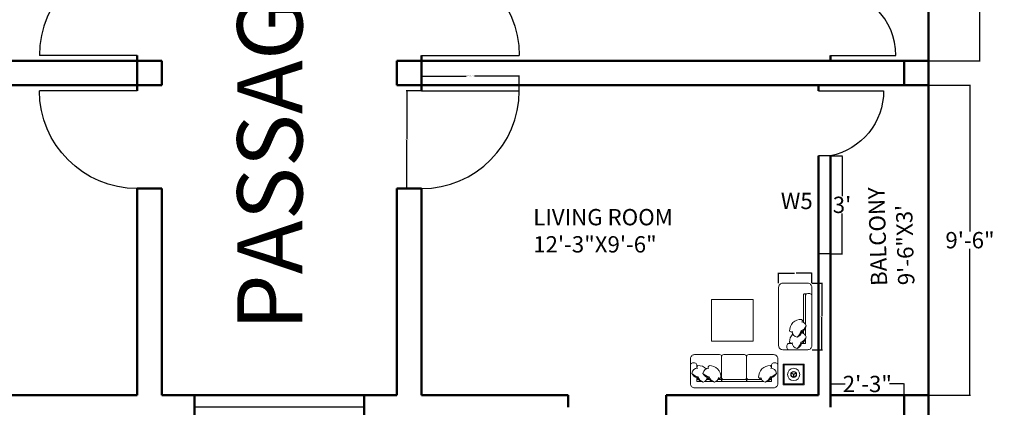
# Model space of a CAD drawing. Units: inches. Extents: x -173 to 545, y -746 to 104.
# Tile 20 of 32: x 168 to 530, y -463 to -321. Entities that reach past the tile are written whole.
import ezdxf

# ---------------------------------------------------------------- set-up
doc = ezdxf.new("R2010")
doc.units = ezdxf.units.IN
doc.header["$MEASUREMENT"] = 0
for name, color, linetype, lineweight in [('A-ANNO-DIMS', 2, 'Continuous', 18), ('A-ANNO-TEXT', 7, 'Continuous', 18), ('A-AREA-IDEN', 7, 'Continuous', 18), ('A-DOOR', 4, 'Continuous', 25), ('A-FURN', 8, 'Continuous', 18), ('A-GLAZ', 3, 'Continuous', 25), ('A-WALL', 7, 'Continuous', 50)]:
    doc.layers.add(name, color=color, linetype=linetype, lineweight=lineweight)
doc.styles.get("Standard").update_dxf_attribs({"font": 'arial.ttf'})
doc.dimstyles.get("Standard").update_dxf_attribs({"dimtxt": 0.18, "dimasz": 0.18, "dimexe": 0.18, "dimexo": 0.0625, "dimgap": 0.09, "dimtad": 0, "dimtih": 1, "dimtoh": 1, "dimdec": 0, "dimzin": 0, "dimdsep": 46, "dimlunit": 3, "dimtxsty": 'Standard', "dimcen": 0.09, "dimadec": 0, "dimazin": 0, "dimtfac": 1, "dimtdec": 0, "dimtofl": 0, "dimtmove": 0, "dimatfit": 3, "dimfxl": 1, "dimtolj": 1, "dimtzin": 0, "dimarcsym": 0})

# ---------------------------------------------------------------- blocks, each defined once
blk = doc.blocks.new('*D8')
at = {"layer": 'A-ANNO-DIMS', "color": 0, "lineweight": -2, "transparency": 16777216}
for p, q in [((501.86, -221.86), (520.82, -221.86)), ((520.64, -222.04), (520.64, -275.71)), ((520.64, -335.68), (520.64, -282.02)), ((501.86, -335.86), (520.82, -335.86))]:
    blk.add_line(p, q, dxfattribs=at)
at = {"layer": 'A-ANNO-DIMS', "color": 0, "transparency": 16777216}
for points in [[(520.61, -222.04), (520.67, -222.04), (520.64, -221.86)], [(520.61, -335.68), (520.67, -335.68), (520.64, -335.86)]]:
    blk.add_solid(points, dxfattribs=at)
at = {"layer": 'Defpoints', "color": 0, "transparency": 16777216}
for p in [(501.8, -221.86), (501.8, -335.86), (520.64, -335.86)]:
    blk.add_point(p, dxfattribs=at)
at = {"layer": 'A-ANNO-DIMS', "color": 0, "transparency": 16777216, "insert": (520.64, -278.86), "char_height": 6, "attachment_point": 5}
blk.add_mtext('\\A1;9\'-6"', dxfattribs=at)
blk = doc.blocks.new('*D13')
at = {"layer": 'A-ANNO-DIMS', "color": 0, "lineweight": -2, "transparency": 16777216}
for p, q in [((465.86, -370.86), (470.17, -370.86)), ((469.99, -371.04), (469.99, -385.71)), ((469.99, -406.68), (469.99, -392.02)), ((465.86, -406.86), (470.17, -406.86))]:
    blk.add_line(p, q, dxfattribs=at)
at = {"layer": 'A-ANNO-DIMS', "color": 0, "transparency": 16777216}
for points in [[(469.96, -371.04), (470.02, -371.04), (469.99, -370.86)], [(469.96, -406.68), (470.02, -406.68), (469.99, -406.86)]]:
    blk.add_solid(points, dxfattribs=at)
at = {"layer": 'Defpoints', "color": 0, "transparency": 16777216}
for p in [(465.8, -370.86), (465.8, -406.86), (469.99, -406.86)]:
    blk.add_point(p, dxfattribs=at)
at = {"layer": 'A-ANNO-DIMS', "color": 0, "transparency": 16777216, "insert": (469.99, -388.86), "char_height": 6, "attachment_point": 5}
blk.add_mtext("\\A1;3'", dxfattribs=at)
blk = doc.blocks.new('*D17')
at = {"layer": 'A-ANNO-DIMS', "color": 0, "lineweight": -2, "transparency": 16777216}
for p, q in [((465.8, -458.8), (465.8, -454.59)), ((465.98, -454.77), (471.19, -454.77)), ((492.62, -454.77), (487.42, -454.77)), ((492.8, -458.8), (492.8, -454.59))]:
    blk.add_line(p, q, dxfattribs=at)
at = {"layer": 'A-ANNO-DIMS', "color": 0, "transparency": 16777216}
for points in [[(465.98, -454.74), (465.98, -454.8), (465.8, -454.77)], [(492.62, -454.74), (492.62, -454.8), (492.8, -454.77)]]:
    blk.add_solid(points, dxfattribs=at)
at = {"layer": 'Defpoints', "color": 0, "transparency": 16777216}
for p in [(492.8, -454.77), (465.8, -458.86), (492.8, -458.86)]:
    blk.add_point(p, dxfattribs=at)
at = {"layer": 'A-ANNO-DIMS', "color": 0, "transparency": 16777216, "insert": (479.3, -454.77), "char_height": 6, "attachment_point": 5}
blk.add_mtext('\\A1;2\'-3"', dxfattribs=at)
blk = doc.blocks.new('*D18')
at = {"layer": 'A-ANNO-DIMS', "color": 0, "lineweight": -2, "transparency": 16777216}
for p, q in [((501.86, -344.86), (517.24, -344.86)), ((517.06, -345.04), (517.06, -398.71)), ((517.06, -458.68), (517.06, -405.02)), ((501.86, -458.86), (517.24, -458.86))]:
    blk.add_line(p, q, dxfattribs=at)
at = {"layer": 'A-ANNO-DIMS', "color": 0, "transparency": 16777216}
for points in [[(517.03, -345.04), (517.09, -345.04), (517.06, -344.86)], [(517.03, -458.68), (517.09, -458.68), (517.06, -458.86)]]:
    blk.add_solid(points, dxfattribs=at)
at = {"layer": 'Defpoints', "color": 0, "transparency": 16777216}
for p in [(501.8, -344.86), (501.8, -458.86), (517.06, -458.86)]:
    blk.add_point(p, dxfattribs=at)
at = {"layer": 'A-ANNO-DIMS', "color": 0, "transparency": 16777216, "insert": (517.06, -401.86), "char_height": 6, "attachment_point": 5}
blk.add_mtext('\\A1;9\'-6"', dxfattribs=at)
blk = doc.blocks.new('DAY BED1')
at = {"color": 0}
blk.add_line((0.3, 0.25), (0.225, 0.255), dxfattribs=at)
blk.add_lwpolyline([(-0.3, 0, -0.414214), (-0.4, 0.1), (-0.4, 0.1, 0.317837), (-0.4, 0.1, -0.414214), (-0.4, 0.1), (-0.4, 0.1, 1.186185), (-0.4, 0.1, -0.414214), (-0.4, 0.1), (-0.4, 1.5, -0.414214), (-0.3, 1.6), (0.3, 1.6, -0.414214), (0.4, 1.5), (0.4, 0.1, -0.414214), (0.3, 0)], format="xyb", close=True, dxfattribs=at)
for points in [[(-0.073, 1.45), (-0.15, 1.45, -0.414214), (-0.2, 1.5), (-0.2, 1.55, -0.414214), (-0.15, 1.6)], [(-0.073, 1.45, 0.165541), (-0.139, 1.419, 0.200231), (-0.058, 1.221, 0.121523)], [(-0.076, 1.425, -0.356772), (0.05, 1.568, -0.249542), (0.154, 1.438, 9.61688)], [(0.05, 1.568, -0.14773), (0.136, 1.422, -0.213343), (0.262, 1.293, -0.178662)], [(0.143, 1.442, -0.306663), (0.262, 1.293, -0.30633), (0.154, 1.196, 0.872847)], [(0.25, 1.345), (0.25, 1.45), (0.152, 1.45, -0.414214)], [(0.2, 1.412), (0.2, 1.43, -0.414214), (0.22, 1.45), (0.23, 1.45, -0.414214), (0.25, 1.43)], [(0.25, 1.43), (0.25, 1.345, -0.414214)], [(-0.076, 1.156, -0.356772), (0.05, 1.299, -0.249542), (0.154, 1.169, 9.61688)], [(0.05, 1.299, -0.14773), (0.136, 1.153, -0.213343), (0.262, 1.024, -0.178662)], [(0.168, 1.163, 0.071865), (0.187, 1.205, -7.115464)], [(0.2, 1.142), (0.2, 1.211, -0.414214)], [(0.25, 1.262), (0.25, 1.075, -0.414214)], [(-0.073, 1.181, 0.165541), (-0.139, 1.15, 0.425989), (0.148, 0.869, 0.121523), (0.187, 0.936, -7.115464)], [(0.143, 1.173, -0.306663), (0.262, 1.024, -0.30633), (0.154, 0.926, 0.872847)], [(0.25, 0.992), (0.25, 0.275, -0.414214), (0.23, 0.255), (0.22, 0.255, -0.414214), (0.2, 0.275), (0.2, 0.942, -0.414214)], [(0.25, 0.377), (0.25, 0.3, 0.414214), (0.3, 0.25), (0.35, 0.25, 0.414214), (0.4, 0.3)]]:
    blk.add_lwpolyline(points, format="xyb", dxfattribs=at)
for points in [[(0.25, 1.075), (0.25, 1.262)], [(0.25, 0.377), (0.25, 0.992)]]:
    blk.add_lwpolyline(points, dxfattribs=at)
blk = doc.blocks.new('DOOR-24')
blk.add_line((24, 0), (24, 24))
blk.add_arc((24, 0), 24, 90, 180)
blk = doc.blocks.new('DOOR-36')
blk.add_line((36, 0), (0, 0))
blk.add_arc((36, 0), 36, 90, 180)
blk = doc.blocks.new('DOOR-24-OFFSET')
blk.add_line((24, 24), (0, 24))
blk.add_arc((24.52, 24), 24.52, 180, 258.1877)
blk = doc.blocks.new('*D50')
at = {"layer": 'A-ANNO-DIMS', "color": 0, "lineweight": -2, "transparency": 16777216}
for p, q in [((458.97, -417.69), (462.76, -417.69)), ((462.58, -417.87), (462.58, -429.75)), ((462.58, -442), (462.58, -430.12)), ((458.97, -442.18), (462.76, -442.18))]:
    blk.add_line(p, q, dxfattribs=at)
at = {"layer": 'A-ANNO-DIMS', "color": 0, "transparency": 16777216}
for points in [[(462.55, -417.87), (462.61, -417.87), (462.58, -417.69)], [(462.55, -442), (462.61, -442), (462.58, -442.18)]]:
    blk.add_solid(points, dxfattribs=at)
at = {"layer": 'Defpoints', "color": 0, "transparency": 16777216}
for p in [(458.91, -417.69), (458.91, -442.18), (462.58, -442.18)]:
    blk.add_point(p, dxfattribs=at)
at = {"layer": 'A-ANNO-DIMS', "color": 0, "transparency": 16777216, "insert": (462.58, -429.94), "char_height": 0.18, "attachment_point": 5}
blk.add_mtext('\\A1;DAY BED 2\'-0 1/2"', dxfattribs=at)
blk = doc.blocks.new('*D51')
at = {"layer": 'A-ANNO-DIMS', "color": 0, "lineweight": -2, "transparency": 16777216}
for p, q in [((446.67, -417.63), (446.67, -413.84)), ((446.85, -414.02), (452.47, -414.02)), ((458.73, -414.02), (453.11, -414.02)), ((458.91, -417.63), (458.91, -413.84))]:
    blk.add_line(p, q, dxfattribs=at)
at = {"layer": 'A-ANNO-DIMS', "color": 0, "transparency": 16777216}
for points in [[(446.85, -413.99), (446.85, -414.05), (446.67, -414.02)], [(458.73, -413.99), (458.73, -414.05), (458.91, -414.02)]]:
    blk.add_solid(points, dxfattribs=at)
at = {"layer": 'Defpoints', "color": 0, "transparency": 16777216}
for p in [(458.91, -414.02), (446.67, -417.69), (458.91, -417.69)]:
    blk.add_point(p, dxfattribs=at)
at = {"layer": 'A-ANNO-DIMS', "color": 0, "transparency": 16777216, "insert": (452.79, -414.02), "char_height": 0.18, "attachment_point": 5}
blk.add_mtext('\\A1;1\'-0"', dxfattribs=at)
blk = doc.blocks.new('*D54')
at = {"layer": 'A-ANNO-DIMS', "color": 0, "lineweight": -2, "transparency": 16777216}
for p, q in [((315.3, -346.8), (315.3, -341.28)), ((315.48, -341.46), (331.79, -341.46)), ((351.12, -341.46), (334.81, -341.46)), ((351.3, -346.8), (351.3, -341.28))]:
    blk.add_line(p, q, dxfattribs=at)
at = {"layer": 'A-ANNO-DIMS', "color": 0, "transparency": 16777216}
for points in [[(315.48, -341.43), (315.48, -341.49), (315.3, -341.46)], [(351.12, -341.43), (351.12, -341.49), (351.3, -341.46)]]:
    blk.add_solid(points, dxfattribs=at)
at = {"layer": 'Defpoints', "color": 0, "transparency": 16777216}
for p in [(315.3, -341.46), (315.3, -346.86), (351.3, -346.86)]:
    blk.add_point(p, dxfattribs=at)
at = {"layer": 'A-ANNO-DIMS', "color": 0, "transparency": 16777216, "insert": (333.3, -341.46), "char_height": 0.18, "attachment_point": 5}
blk.add_mtext('\\A1;ENTRY DOOR 3\'-0" TYP.', dxfattribs=at)
blk = doc.blocks.new('*D55')
at = {"layer": 'A-ANNO-DIMS', "color": 0, "lineweight": -2, "transparency": 16777216}
for p, q in [((315.24, -346.86), (309.72, -346.86)), ((309.9, -347.04), (309.9, -364.68)), ((309.9, -382.68), (309.9, -365.04)), ((315.24, -382.86), (309.72, -382.86))]:
    blk.add_line(p, q, dxfattribs=at)
at = {"layer": 'A-ANNO-DIMS', "color": 0, "transparency": 16777216}
for points in [[(309.87, -347.04), (309.93, -347.04), (309.9, -346.86)], [(309.87, -382.68), (309.93, -382.68), (309.9, -382.86)]]:
    blk.add_solid(points, dxfattribs=at)
at = {"layer": 'Defpoints', "color": 0, "transparency": 16777216}
for p in [(315.3, -346.86), (309.9, -382.86), (315.3, -382.86)]:
    blk.add_point(p, dxfattribs=at)
at = {"layer": 'A-ANNO-DIMS', "color": 0, "transparency": 16777216, "insert": (309.9, -364.86), "char_height": 0.18, "attachment_point": 5}
blk.add_mtext('\\A1;3\'-0" TYP.', dxfattribs=at)

msp = doc.modelspace()

# ---------------------------------------------------------------- linework, layer by layer
at = {"layer": 'A-DOOR'}
msp.add_line((294.3, -463.36), (231.8, -463.36), dxfattribs=at)
at = {"layer": 'A-FURN'}
for p, q in [((452.19, -451.3), (451.26, -450.76)), ((452.24, -451.21), (451.3, -450.67)), ((452.17, -451.26), (452.17, -452.33)), ((452.19, -451.21), (453.12, -450.67)), ((452.24, -451.3), (453.17, -450.76)), ((452.26, -451.26), (452.26, -452.33))]:
    msp.add_line(p, q, dxfattribs=at)
at = {"layer": 'A-FURN', "ltscale": 0.03}
for points in [[(421.99, -423.71), (437.3, -423.71), (437.3, -439.01), (421.99, -439.01)], [(456.04, -447.43), (448.39, -447.43), (448.39, -455.08), (456.04, -455.08)]]:
    msp.add_lwpolyline(points, close=True, dxfattribs=at)
msp.add_lwpolyline([(446.38, -445.5, 0.414214), (444.85, -443.97), (435.67, -443.97, 0.414214), (434.9, -444.73, 0.414214), (434.14, -443.97), (426.49, -443.97, 0.414214), (425.72, -444.73, 0.414214), (424.96, -443.97), (415.78, -443.97, 0.414214), (414.25, -445.5), (414.25, -454.68, 0.414214), (415.78, -456.21), (444.85, -456.21, 0.414214), (446.38, -454.68)], format="xyb", close=True, dxfattribs=at)
at = {"layer": 'A-FURN'}
for points in [[(424.96, -453.15, 0.414214), (425.72, -452.38), (425.72, -444.73, 0.414214)], [(435.67, -453.15, -0.414214), (434.9, -452.38), (434.9, -444.73, -0.414214)], [(416.54, -448.98), (416.54, -447.79, 0.414214), (415.78, -447.03), (415.01, -447.03, 0.414214), (414.25, -447.79)], [(416.92, -448.93, 0.356772), (414.73, -450.86, 0.249542), (416.72, -452.45, -9.61688)], [(416.54, -448.98, -0.165541), (417.01, -447.97, -0.200231), (420.05, -449.2, -0.121523)], [(421.05, -448.93, 0.356772), (418.85, -450.86, 0.249542), (420.84, -452.45, -9.61688)], [(420.66, -448.98, -0.165541), (421.13, -447.97, -0.425989), (425.43, -452.35, -0.121523), (424.41, -452.95, 7.115464)], [(444.09, -448.98, 0.165541), (443.61, -447.97, 0.425989), (439.32, -452.35, 0.121523), (440.34, -452.95, -7.115464)], [(443.7, -448.93, -0.356772), (445.89, -450.86, -0.249542), (443.91, -452.45, 9.61688)], [(446.38, -447.79, 0.414214), (445.61, -447.03), (444.85, -447.03, 0.414214), (444.08, -447.79), (444.08, -448.98)], [(414.73, -450.86, 0.14773), (416.97, -452.17, 0.213343), (418.94, -454.1, 0.178662)], [(418.15, -453.91), (416.54, -453.91), (416.54, -452.41, 0.414214)], [(416.66, -452.28, 0.306663), (418.94, -454.1, 0.30633), (420.43, -452.44, -0.872847)], [(418.85, -450.86, 0.14773), (421.09, -452.17, 0.213343), (423.06, -454.1, 0.178662)], [(420.93, -452.65, -0.071865), (420.29, -452.95, 7.115464)], [(420.78, -452.28, 0.306663), (423.06, -454.1, 0.30633), (424.55, -452.44, -0.872847)], [(426.49, -453.15, -0.414214), (425.72, -452.38)], [(434.14, -453.15, 0.414214), (434.9, -452.38)], [(443.96, -452.28, -0.306663), (441.68, -454.1, -0.30633), (440.19, -452.44, 0.872847)], [(445.89, -450.86, -0.14773), (443.66, -452.17, -0.213343), (441.68, -454.1, -0.178662)], [(417.12, -453.15), (416.85, -453.15, 0.414214), (416.54, -453.45), (416.54, -453.61, 0.414214), (416.85, -453.91)], [(416.85, -453.91), (418.15, -453.91, 0.414214)], [(419.42, -453.91), (422.27, -453.91, 0.414214)], [(421.25, -453.15), (420.19, -453.15, 0.414214)], [(423.54, -453.91), (425.42, -453.91, 0.414214), (425.72, -453.61), (425.72, -453.45, 0.414214), (425.42, -453.15), (424.31, -453.15, 0.414214)], [(441.2, -453.91), (435.21, -453.91, -0.414214), (434.9, -453.61), (434.9, -453.45, -0.414214), (435.21, -453.15), (440.43, -453.15, -0.414214)], [(443.78, -453.91), (442.47, -453.91, -0.414214)], [(443.5, -453.15), (443.78, -453.15, -0.414214), (444.08, -453.45), (444.08, -453.61, -0.414214), (443.78, -453.91)]]:
    msp.add_lwpolyline(points, format="xyb", dxfattribs=at)
msp.add_lwpolyline([(448.7, -447.74), (455.73, -447.74), (455.73, -454.77), (448.7, -454.77)], close=True, dxfattribs=at)
for points in [[(444.08, -452.41), (444.08, -453.91), (442.47, -453.91)], [(422.27, -453.91), (419.42, -453.91)], [(441.2, -453.91), (423.54, -453.91)]]:
    msp.add_lwpolyline(points, dxfattribs=at)
msp.add_lwpolyline([(426.03, -453.91), (434.6, -453.91, 0.414214), (434.9, -453.61), (434.9, -453.45, 0.414214), (434.6, -453.15), (426.03, -453.15, 0.414214), (425.72, -453.45), (425.72, -453.61, 0.414214)], format="xyb", close=True, dxfattribs=at)
for radius in [2.26, 1.08, 0.968]:
    msp.add_circle((452.21, -451.26), radius, dxfattribs=at)
at = {"layer": 'A-GLAZ'}
for p, q in [((465.8, -370.86), (461.3, -370.86)), ((465.8, -406.86), (461.3, -406.86))]:
    msp.add_line(p, q, dxfattribs=at)
at = {"layer": 'A-WALL'}
for p, q in [((501.8, 7.64), (501.8, -697.36)), ((24.3, -335.86), (219.8, -335.86)), ((210.8, -333.86), (210.8, -344.86)), ((219.8, -335.86), (219.8, -344.86)), ((306.3, -335.86), (306.3, -344.86)), ((306.3, -335.86), (501.8, -335.86)), ((315.3, -333.86), (315.3, -344.86)), ((465.8, -333.86), (465.8, -335.86)), ((492.8, -335.86), (492.8, -344.86)), ((24.3, -344.86), (219.8, -344.86)), ((210.8, -344.86), (210.8, -346.86)), ((306.3, -344.86), (501.8, -344.86)), ((315.3, -344.86), (315.3, -346.86)), ((461.3, -344.86), (461.3, -346.86)), ((461.3, -370.86), (461.3, -458.86)), ((465.8, -370.86), (465.8, -463.36)), ((210.8, -382.86), (219.8, -382.86)), ((210.8, -382.86), (210.8, -458.86)), ((219.8, -382.86), (219.8, -458.86)), ((306.3, -382.86), (306.3, -458.86)), ((315.3, -382.86), (306.3, -382.86)), ((315.3, -382.86), (315.3, -458.86)), ((156.8, -458.86), (210.8, -458.86)), ((219.8, -458.86), (306.3, -458.86)), ((231.8, -458.86), (231.8, -467.86)), ((294.3, -458.86), (294.3, -467.86)), ((315.3, -458.86), (369.3, -458.86)), ((369.3, -458.86), (369.3, -463.36)), ((405.3, -458.86), (405.3, -505.36)), ((405.3, -458.86), (461.3, -458.86)), ((465.8, -458.86), (501.8, -458.86)), ((492.8, -458.86), (492.8, -505.36))]:
    msp.add_line(p, q, dxfattribs=at)

# ---------------------------------------------------------------- block references
at = {"layer": 'A-DOOR'}
msp.add_blockref('DOOR-36', (174.8, -333.86), dxfattribs=at)
at = {"layer": 'A-DOOR', "extrusion": (0, 0, -1), "zscale": -1}
for name, p in [('DOOR-36', (-351.3, -333.86)), ('DOOR-24-OFFSET', (-485.3, -370.86))]:
    msp.add_blockref(name, p, dxfattribs=at)
at = {"layer": 'A-DOOR'}
for name, p, rotation in [('DOOR-24', (465.8, -309.86), 270.0000000000001), ('DOOR-36', (351.3, -346.86), 180)]:
    msp.add_blockref(name, p, dxfattribs=dict(at, rotation=rotation))
at = {"layer": 'A-DOOR', "extrusion": (0, 0, -1), "zscale": -1, "rotation": 180}
msp.add_blockref('DOOR-36', (-174.8, -346.86), dxfattribs=at)
at = {"layer": 'A-FURN', "ltscale": 0.03, "xscale": -15.30180482051142, "yscale": 15.30180482051142, "zscale": 15.30180482051142, "rotation": 180}
msp.add_blockref('DAY BED1', (452.79, -417.69), dxfattribs=at)

# ---------------------------------------------------------------- texts
at = {"layer": 'A-ANNO-TEXT', "insert": (447.49, -384.42), "char_height": 6, "attachment_point": 1}
msp.add_mtext('W5', dxfattribs=at)
at = {"layer": 'A-AREA-IDEN', "attachment_point": 1}
for s, insert, char_height, rotation in [('PASSAGE', (247.55, -435.15), 24, 90), ('BALCONY\\P9\'-6"X3\'', (480.65, -418.8), 6, 91.7171)]:
    msp.add_mtext(s, dxfattribs=dict(at, insert=insert, char_height=char_height, rotation=rotation))
at = {"layer": 'A-AREA-IDEN', "insert": (356.42, -390.39), "char_height": 6, "attachment_point": 1}
msp.add_mtext('LIVING ROOM\\P12\'-3"X9\'-6"', dxfattribs=at)

# ---------------------------------------------------------------- dimensions: what is measured, and where the dimension line sits
at = {"layer": 'A-ANNO-DIMS'}
for base, p1, p2, picture, middle in [((520.64, -335.86), (501.8, -221.86), (501.8, -335.86), '*D8', (520.64, -278.86)), ((517.06, -458.86), (501.8, -344.86), (501.8, -458.86), '*D18', (517.06, -401.86)), ((469.99, -406.86), (465.8, -370.86), (465.8, -406.86), '*D13', (469.99, -388.86))]:
    dim = msp.add_linear_dim(base=base, p1=p1, p2=p2, angle=90, dimstyle='Standard', override={"dimtxt": 6, "dimclrd": 0, "dimclre": 0, "dimclrt": 0}, dxfattribs=at)
    dim.commit()
    dim.dimension.update_dxf_attribs({"geometry": picture, "text_midpoint": middle})
for base, p1, p2, angle, text, picture, middle in [((315.3, -341.46), (351.3, -346.86), (315.3, -346.86), 180, 'ENTRY DOOR <> TYP.', '*D54', (333.3, -341.46)), ((309.9, -382.86), (315.3, -346.86), (315.3, -382.86), 270, '<> TYP.', '*D55', (309.9, -364.86)), ((462.58, -442.18), (458.91, -417.69), (458.91, -442.18), 270, 'DAY BED <>', '*D50', (462.58, -429.94))]:
    dim = msp.add_linear_dim(base=base, p1=p1, p2=p2, angle=angle, text=text, dimstyle='Standard', override={"dimdec": 1, "dimlfac": 1, "dimrnd": 0, "dimzin": 1, "dimdsep": 46, "dimlunit": 4, "dimfrac": 2}, dxfattribs=at)
    dim.commit()
    dim.dimension.update_dxf_attribs({"geometry": picture, "text_midpoint": middle})
for base, p1, p2, override, picture, middle in [((458.91, -414.02), (446.67, -417.69), (458.91, -417.69), {"dimdec": 1, "dimlfac": 1, "dimrnd": 0, "dimzin": 1, "dimdsep": 46, "dimlunit": 4, "dimfrac": 2}, '*D51', (452.79, -414.02)), ((492.8, -454.77), (465.8, -458.86), (492.8, -458.86), {"dimtxt": 6, "dimclrd": 0, "dimclre": 0, "dimclrt": 0}, '*D17', (479.3, -454.77))]:
    dim = msp.add_linear_dim(base=base, p1=p1, p2=p2, dimstyle='Standard', override=override, dxfattribs=at)
    dim.commit()
    dim.dimension.update_dxf_attribs({"geometry": picture, "text_midpoint": middle})

doc.saveas('drawing.dxf')
